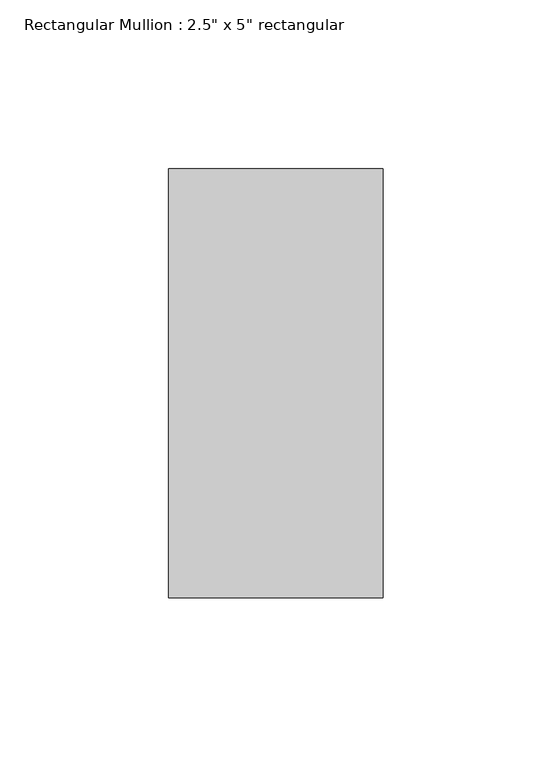
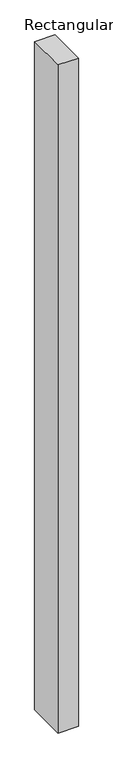
"""IFC4 building model written with IfcOpenShell, lengths in millimetres: member geometry."""

from ifc_helpers import new_model, si_unit, frame, origin, place, context, project, spatial, polyline, outline, extrude, source, transform, mapped, element, save


def member_c841a703(model_context):
    return source(origin(), model_context, "Body", "SweptSolid", [
        extrude(outline(polyline([(0.0, 63.5), (0.0, -63.5), (-63.5, -63.5), (-63.5, 63.5), (0.0, 63.5)])), frame((0.0, 0.0, -2214.7649104), z_axis=(0.0, 0.0, 1.0), x_axis=(1.0, 0.0, 0.0)), (0.0, 0.0, 1.0), 2214.7649104),
    ])


if __name__ == "__main__":
    model = new_model("IFC4")
    model_context = context("Model", 3, world=origin())
    ifc_project = project(units=[si_unit("LENGTHUNIT", "METRE", prefix="MILLI")], contexts=[model_context])
    site = spatial("IfcSite", under=ifc_project)
    building = spatial("IfcBuilding", under=site)
    placement = place(None, origin())
    member_shape = member_c841a703(model_context)
    element("IfcMember", 1, ObjectType="Rectangular Mullion : 2.5\" x 5\" rectangular", at=placement, inside=building, context=model_context, shape_type="MappedRepresentation", body=[
        mapped(member_shape, transform((0.0, 0.0, 0.0), x_axis=(1.0, 0.0, 0.0), y_axis=(0.0, 1.0, 0.0), z_axis=(0.0, 0.0, 1.0))),
    ])
    save(model, "model.ifc")

# Revit data of these elements
# Type "Rectangular Mullion : 2.5\" x 5\" rectangular"
#   built-in parameter 1007304 = 0.416667 (stored number, unit not read)
#   built-in parameter 1007301 = 0.104167 (stored number, unit not read)
#   built-in parameter 1007300 = 0.104167 (stored number, unit not read)
# Element 1 (IfcMember, "Rectangular Mullion : 2.5\" x 5\" rectangular")
#   Materials on its faces: "Aluminum"
# Materials
#   "Aluminum": class "Metal", colour RGB 247 247 247, transparency 0, Description = "Aluminum 6061", Cost = 0
